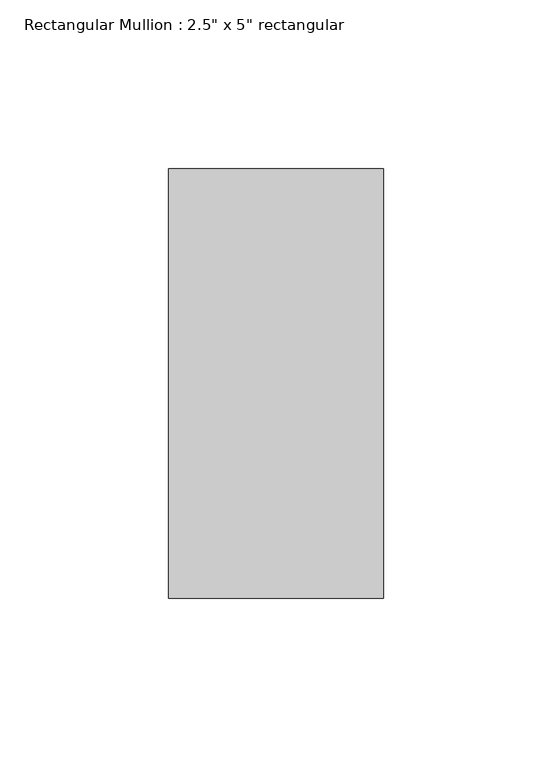
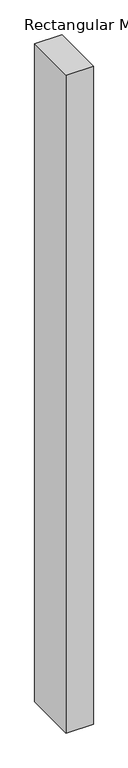
"""IFC4 building model written with IfcOpenShell, lengths in millimetres: member geometry."""

from ifc_helpers import new_model, si_unit, frame, origin, place, context, project, spatial, polyline, outline, extrude, source, transform, mapped, element, save


def member_46459143(model_context):
    return source(origin(), model_context, "Body", "SweptSolid", [
        extrude(outline(polyline([(0.0, 63.5), (0.0, -63.5), (-63.5, -63.5), (-63.5, 63.5), (0.0, 63.5)])), frame((0.0, 0.0, -1623.9353791), z_axis=(0.0, 0.0, 1.0), x_axis=(1.0, 0.0, 0.0)), (0.0, 0.0, 1.0), 1623.9353791),
    ])


if __name__ == "__main__":
    model = new_model("IFC4")
    model_context = context("Model", 3, world=origin())
    ifc_project = project(units=[si_unit("LENGTHUNIT", "METRE", prefix="MILLI")], contexts=[model_context])
    site = spatial("IfcSite", under=ifc_project)
    building = spatial("IfcBuilding", under=site)
    placement = place(None, origin())
    member_shape = member_46459143(model_context)
    element("IfcMember", 1, ObjectType="Rectangular Mullion : 2.5\" x 5\" rectangular", at=placement, inside=building, context=model_context, shape_type="MappedRepresentation", body=[
        mapped(member_shape, transform((0.0, 0.0, 0.0), x_axis=(1.0, 0.0, 0.0), y_axis=(0.0, 1.0, 0.0), z_axis=(0.0, 0.0, 1.0))),
    ])
    save(model, "model.ifc")

# Revit data of these elements
# Type "Rectangular Mullion : 2.5\" x 5\" rectangular"
#   built-in parameter 1007304 = 0.416667 (stored number, unit not read)
#   built-in parameter 1007301 = 0.104167 (stored number, unit not read)
#   built-in parameter 1007300 = 0.104167 (stored number, unit not read)
# Element 1 (IfcMember, "Rectangular Mullion : 2.5\" x 5\" rectangular")
#   Materials on its faces: "Aluminum"
# Materials
#   "Aluminum": class "Metal", colour RGB 247 247 247, transparency 0, Description = "Aluminum 6061", Cost = 0
